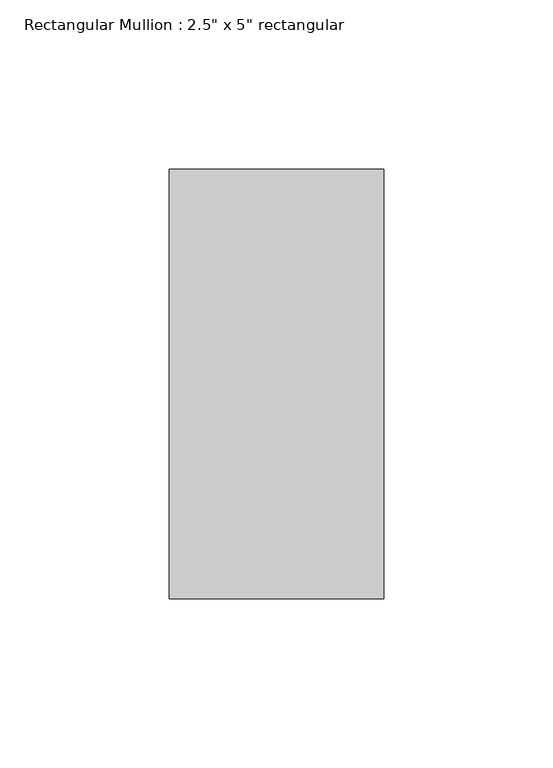
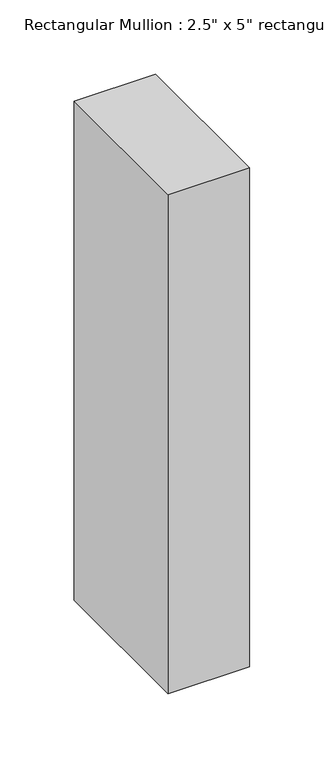
"""IFC4 building model written with IfcOpenShell, lengths in millimetres: member geometry."""

from ifc_helpers import new_model, si_unit, frame, origin, place, context, project, spatial, polyline, outline, extrude, source, transform, mapped, element, save


def member_34d525fb(model_context):
    return source(origin(), model_context, "Body", "SweptSolid", [
        extrude(outline(polyline([(31.75, 63.5), (31.75, -63.5), (-31.75, -63.5), (-31.75, 63.5), (31.75, 63.5)])), frame((0.0, 0.0, -410.6333333), z_axis=(0.0, 0.0, 1.0), x_axis=(1.0, 0.0, 0.0)), (0.0, 0.0, 1.0), 410.6333333),
    ])


if __name__ == "__main__":
    model = new_model("IFC4")
    model_context = context("Model", 3, world=origin())
    ifc_project = project(units=[si_unit("LENGTHUNIT", "METRE", prefix="MILLI")], contexts=[model_context])
    site = spatial("IfcSite", under=ifc_project)
    building = spatial("IfcBuilding", under=site)
    placement = place(None, origin())
    member_shape = member_34d525fb(model_context)
    element("IfcMember", 1, ObjectType="Rectangular Mullion : 2.5\" x 5\" rectangular", at=placement, inside=building, context=model_context, shape_type="MappedRepresentation", body=[
        mapped(member_shape, transform((0.0, 0.0, 0.0), x_axis=(1.0, 0.0, 0.0), y_axis=(0.0, 1.0, 0.0), z_axis=(0.0, 0.0, 1.0))),
    ])
    save(model, "model.ifc")

# Revit data of these elements
# Type "Rectangular Mullion : 2.5\" x 5\" rectangular"
#   built-in parameter 1007304 = 0.416667 (stored number, unit not read)
#   built-in parameter 1007301 = 0.104167 (stored number, unit not read)
#   built-in parameter 1007300 = 0.104167 (stored number, unit not read)
